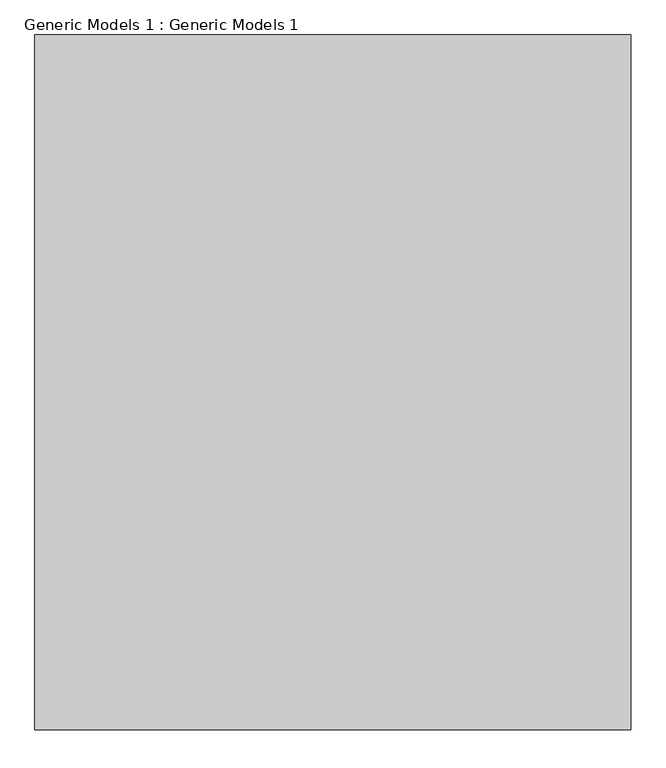
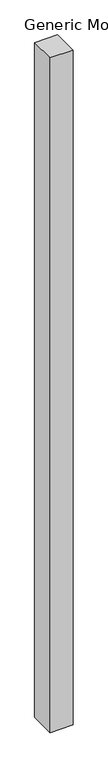
"""IFC4 building model written with IfcOpenShell, lengths in millimetres: proxy geometry, Generic Models 1 : Generic Models 1."""

from ifc_helpers import new_model, si_unit, frame, origin, place, context, project, spatial, polyline, outline, extrude, source, transform, mapped, element, save


def generic_models_1_generic_models_1_b762b88f(model_context):
    return source(origin(), model_context, "Body", "SweptSolid", [
        extrude(outline(polyline([(-12143.6022803, -14078.0808221), (-12143.6022803, -15903.798497), (-13710.2139216, -15903.798497), (-13710.2139216, -14078.0808221), (-12143.6022803, -14078.0808221)])), frame((0.0, 0.0, 6729.6194038), z_axis=(0.0, 0.0, 1.0), x_axis=(1.0, 0.0, 0.0)), (0.0, 0.0, 1.0), 48743.9805962),
    ])


if __name__ == "__main__":
    model = new_model("IFC4")
    model_context = context("Model", 3, world=origin())
    ifc_project = project(units=[si_unit("LENGTHUNIT", "METRE", prefix="MILLI")], contexts=[model_context])
    site = spatial("IfcSite", under=ifc_project)
    building = spatial("IfcBuilding", under=site)
    placement = place(None, origin())
    generic_models_1_generic_models_1_shape = generic_models_1_generic_models_1_b762b88f(model_context)
    element("IfcBuildingElementProxy", 1, Name="Generic Models 1 : Generic Models 1", ObjectType="Generic Models 1 : Generic Models 1", at=placement, inside=building, context=model_context, shape_type="MappedRepresentation", body=[
        mapped(generic_models_1_generic_models_1_shape, transform((0.0, 0.0, 0.0), x_axis=(1.0, 0.0, 0.0), y_axis=(0.0, 1.0, 0.0), z_axis=(0.0, 0.0, 1.0))),
    ])
    save(model, "model.ifc")
